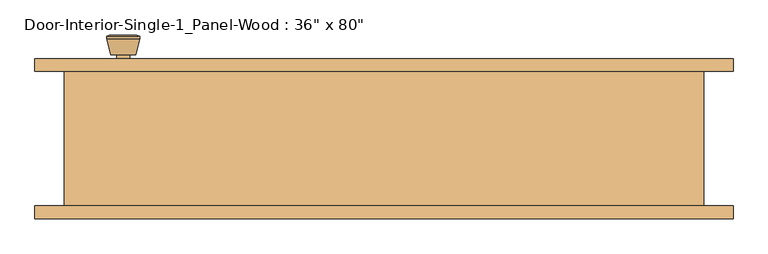
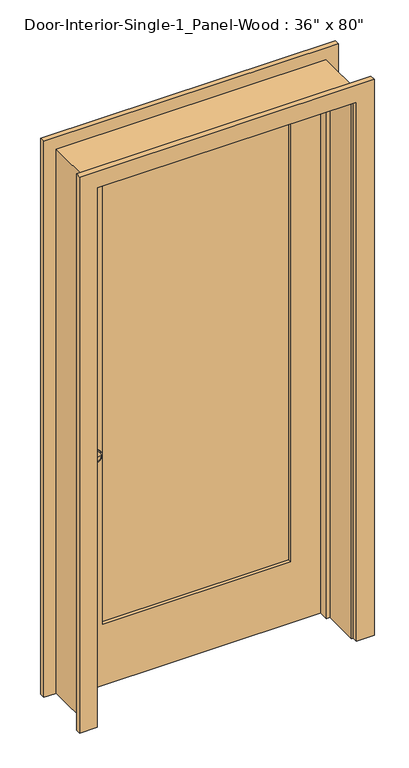
"""IFC4 building model written with IfcOpenShell, lengths in millimetres: door geometry."""

from ifc_helpers import new_model, si_unit, point, frame, frame_2d, origin, place, context, project, spatial, polyline, circle_curve, trimmed, segment, composite_curve, outline, extrude, faceted_brep, source, transform, mapped, element, save
from ifc_brep_helpers import plane_surface, cylinder_surface, revolved_surface, advanced_brep


def door_82825f5f(model_context):
    return source(origin(), model_context, "Body", "SolidModel", [
        advanced_brep(
        [(-393.7, 57.5, 914.4), (-383.7, 57.5, 914.4), (-403.7, 57.5, 914.4), (-373.2241324, 8.5, 914.4), (-393.7, 8.5, 914.4), (-414.1758676, 8.5, 914.4), (-368.7, 10.3278681, 914.4), (-418.7, 10.3278681, 914.4), (-368.7, 13.7915463, 914.4), (-418.7, 13.7915463, 914.4), (-375.063764, 38.5, 914.4), (-412.336236, 38.5, 914.4), (-383.7, 38.5, 914.4), (-403.7, 38.5, 914.4)],
        [
            (0, 1),
            (1, 2, circle_curve(frame((-393.7, 57.5, 914.4), z_axis=(0.0, 1.0, 0.0), x_axis=(-1.0, 0.0, 0.0)), 10.0)),
            (2, 0),
            (2, 1, circle_curve(frame((-393.7, 57.5, 914.4), z_axis=(0.0, 1.0, 0.0), x_axis=(-1.0, 0.0, 0.0)), 10.0)),
            (3, 4),
            (4, 5),
            (5, 3, circle_curve(frame((-393.7, 8.5, 914.4), z_axis=(0.0, -1.0, 0.0), x_axis=(-1.0, 0.0, 0.0)), 20.4758676)),
            (3, 5, circle_curve(frame((-393.7, 8.5, 914.4), z_axis=(0.0, -1.0, 0.0), x_axis=(-1.0, 0.0, 0.0)), 20.4758676)),
            (6, 3),
            (5, 7),
            (7, 6, circle_curve(frame((-393.7, 10.3278681, 914.4), z_axis=(0.0, -1.0, 0.0), x_axis=(-1.0, 0.0, 0.0)), 25.0)),
            (6, 7, circle_curve(frame((-393.7, 10.3278681, 914.4), z_axis=(0.0, -1.0, 0.0), x_axis=(-1.0, 0.0, 0.0)), 25.0)),
            (8, 6),
            (7, 9),
            (9, 8, circle_curve(frame((-393.7, 13.7915463, 914.4), z_axis=(0.0, -1.0, 0.0), x_axis=(-1.0, 0.0, 0.0)), 25.0)),
            (8, 9, circle_curve(frame((-393.7, 13.7915463, 914.4), z_axis=(0.0, -1.0, 0.0), x_axis=(-1.0, 0.0, 0.0)), 25.0)),
            (10, 8),
            (9, 11),
            (11, 10, circle_curve(frame((-393.7, 38.5, 914.4), z_axis=(0.0, -1.0, 0.0), x_axis=(-1.0, 0.0, 0.0)), 18.636236)),
            (10, 11, circle_curve(frame((-393.7, 38.5, 914.4), z_axis=(0.0, -1.0, 0.0), x_axis=(-1.0, 0.0, 0.0)), 18.636236)),
            (12, 10),
            (11, 13),
            (13, 12, circle_curve(frame((-393.7, 38.5, 914.4), z_axis=(0.0, -1.0, 0.0), x_axis=(-1.0, 0.0, 0.0)), 10.0)),
            (12, 13, circle_curve(frame((-393.7, 38.5, 914.4), z_axis=(0.0, -1.0, 0.0), x_axis=(-1.0, 0.0, 0.0)), 10.0)),
            (1, 12),
            (13, 2),
        ],
        [
            plane_surface(frame((-393.7, 57.5, 914.4), z_axis=(0.0, 1.0, 0.0), x_axis=(-1.0, 0.0, 0.0))),
            plane_surface(frame((-393.7, 8.5, 914.4), z_axis=(0.0, -1.0, 0.0), x_axis=(-1.0, 0.0, 0.0))),
            revolved_surface(polyline([(-414.1758676, 8.5, 914.4), (-418.7, 10.3278681, 914.4)]), (-393.7, 57.5, 914.4), (0.0, 1.0, 0.0)),
            cylinder_surface(frame((-393.7, 57.5, 914.4), z_axis=(0.0, 1.0, 0.0), x_axis=(-1.0, 0.0, 0.0)), 25.0),
            revolved_surface(polyline([(-418.7, 13.7915463, 914.4), (-412.336236, 38.5, 914.4)]), (-393.7, 57.5, 914.4), (0.0, 1.0, 0.0)),
            plane_surface(frame((-393.7, 38.5, 914.4), z_axis=(0.0, 1.0, 0.0), x_axis=(-1.0, 0.0, 0.0))),
            cylinder_surface(frame((-393.7, 57.5, 914.4), z_axis=(0.0, 1.0, 0.0), x_axis=(-1.0, 0.0, 0.0)), 10.0),
        ],
        [
            (0, [[1, 2, 3]]),
            (0, [[-3, 4, -1]]),
            (1, [[5, 6, 7]]),
            (1, [[-6, -5, 8]]),
            (2, [[9, -7, 10, 11]]),
            (2, [[-10, -8, -9, 12]]),
            (3, [[13, -11, 14, 15]]),
            (3, [[-14, -12, -13, 16]]),
            (4, [[17, -15, 18, 19]]),
            (4, [[-18, -16, -17, 20]]),
            (5, [[21, -19, 22, 23]]),
            (5, [[-22, -20, -21, 24]]),
            (6, [[25, -23, 26, -2]]),
            (6, [[-26, -24, -25, -4]]),
        ],
    ),
        extrude(outline(composite_curve([segment(trimmed(circle_curve(frame_2d((914.4, -393.7)), 30.0), [point((914.4, -423.7))], [point((914.4, -363.7))], False, "CARTESIAN"), True, "CONTINUOUS"), segment(trimmed(circle_curve(frame_2d((914.4, -393.7)), 30.0), [point((914.4, -363.7))], [point((914.4, -423.7))], False, "CARTESIAN"), True, "CONTINUOUS")], self_intersect=False)), frame((0.0, 57.5, 0.0), z_axis=(0.0, 1.0, 0.0), x_axis=(0.0, 0.0, 1.0)), (0.0, 0.0, 1.0), 6.0),
        advanced_brep(
        [(-393.7, 104.425, 914.4), (-403.7, 104.425, 914.4), (-383.7, 104.425, 914.4), (-373.2241324, 153.425, 914.4), (-414.1758676, 153.425, 914.4), (-393.7, 153.425, 914.4), (-368.7, 151.5971319, 914.4), (-418.7, 151.5971319, 914.4), (-368.7, 148.1334537, 914.4), (-418.7, 148.1334537, 914.4), (-375.063764, 123.425, 914.4), (-412.336236, 123.425, 914.4), (-383.7, 123.425, 914.4), (-403.7, 123.425, 914.4)],
        [
            (0, 1),
            (1, 2, circle_curve(frame((-393.7, 104.425, 914.4), z_axis=(0.0, -1.0, 0.0), x_axis=(-1.0, 0.0, 0.0)), 10.0)),
            (2, 0),
            (2, 1, circle_curve(frame((-393.7, 104.425, 914.4), z_axis=(0.0, -1.0, 0.0), x_axis=(-1.0, 0.0, 0.0)), 10.0)),
            (3, 4, circle_curve(frame((-393.7, 153.425, 914.4), z_axis=(0.0, 1.0, 0.0), x_axis=(-1.0, 0.0, 0.0)), 20.4758676)),
            (4, 5),
            (5, 3),
            (4, 3, circle_curve(frame((-393.7, 153.425, 914.4), z_axis=(0.0, 1.0, 0.0), x_axis=(-1.0, 0.0, 0.0)), 20.4758676)),
            (6, 7, circle_curve(frame((-393.7, 151.5971319, 914.4), z_axis=(0.0, 1.0, 0.0), x_axis=(-1.0, 0.0, 0.0)), 25.0)),
            (7, 4),
            (3, 6),
            (7, 6, circle_curve(frame((-393.7, 151.5971319, 914.4), z_axis=(0.0, 1.0, 0.0), x_axis=(-1.0, 0.0, 0.0)), 25.0)),
            (8, 9, circle_curve(frame((-393.7, 148.1334537, 914.4), z_axis=(0.0, 1.0, 0.0), x_axis=(-1.0, 0.0, 0.0)), 25.0)),
            (9, 7),
            (6, 8),
            (9, 8, circle_curve(frame((-393.7, 148.1334537, 914.4), z_axis=(0.0, 1.0, 0.0), x_axis=(-1.0, 0.0, 0.0)), 25.0)),
            (10, 11, circle_curve(frame((-393.7, 123.425, 914.4), z_axis=(0.0, 1.0, 0.0), x_axis=(-1.0, 0.0, 0.0)), 18.636236)),
            (11, 9),
            (8, 10),
            (11, 10, circle_curve(frame((-393.7, 123.425, 914.4), z_axis=(0.0, 1.0, 0.0), x_axis=(-1.0, 0.0, 0.0)), 18.636236)),
            (12, 13, circle_curve(frame((-393.7, 123.425, 914.4), z_axis=(0.0, 1.0, 0.0), x_axis=(-1.0, 0.0, 0.0)), 10.0)),
            (13, 11),
            (10, 12),
            (13, 12, circle_curve(frame((-393.7, 123.425, 914.4), z_axis=(0.0, 1.0, 0.0), x_axis=(-1.0, 0.0, 0.0)), 10.0)),
            (1, 13),
            (12, 2),
        ],
        [
            plane_surface(frame((-393.7, 104.425, 914.4), z_axis=(0.0, -1.0, 0.0), x_axis=(-1.0, 0.0, 0.0))),
            plane_surface(frame((-393.7, 153.425, 914.4), z_axis=(0.0, 1.0, 0.0), x_axis=(-1.0, 0.0, 0.0))),
            revolved_surface(polyline([(-414.1758676, 153.425, 914.4), (-418.7, 151.5971319, 914.4)]), (-393.7, 104.425, 914.4), (0.0, -1.0, 0.0)),
            cylinder_surface(frame((-393.7, 104.425, 914.4), z_axis=(0.0, -1.0, 0.0), x_axis=(-1.0, 0.0, 0.0)), 25.0),
            revolved_surface(polyline([(-418.7, 148.1334537, 914.4), (-412.336236, 123.425, 914.4)]), (-393.7, 104.425, 914.4), (0.0, -1.0, 0.0)),
            plane_surface(frame((-393.7, 123.425, 914.4), z_axis=(0.0, -1.0, 0.0), x_axis=(-1.0, 0.0, 0.0))),
            cylinder_surface(frame((-393.7, 104.425, 914.4), z_axis=(0.0, -1.0, 0.0), x_axis=(-1.0, 0.0, 0.0)), 10.0),
        ],
        [
            (0, [[1, 2, 3]]),
            (0, [[-3, 4, -1]]),
            (1, [[5, 6, 7]]),
            (1, [[8, -7, -6]]),
            (2, [[9, 10, -5, 11]]),
            (2, [[12, -11, -8, -10]]),
            (3, [[13, 14, -9, 15]]),
            (3, [[16, -15, -12, -14]]),
            (4, [[17, 18, -13, 19]]),
            (4, [[20, -19, -16, -18]]),
            (5, [[21, 22, -17, 23]]),
            (5, [[24, -23, -20, -22]]),
            (6, [[-2, 25, -21, 26]]),
            (6, [[-4, -26, -24, -25]]),
        ],
    ),
        extrude(outline(composite_curve([segment(trimmed(circle_curve(frame_2d((914.4, -393.7)), 30.0), [point((914.4, -423.7))], [point((914.4, -363.7))], False, "CARTESIAN"), True, "CONTINUOUS"), segment(trimmed(circle_curve(frame_2d((914.4, -393.7)), 30.0), [point((914.4, -363.7))], [point((914.4, -423.7))], False, "CARTESIAN"), True, "CONTINUOUS")], self_intersect=False)), frame((0.0, 98.425, 0.0), z_axis=(0.0, 1.0, 0.0), x_axis=(0.0, 0.0, 1.0)), (0.0, 0.0, 1.0), 6.0),
        faceted_brep([(482.6, 98.425, 0.0), (482.6, -104.775, 0.0), (457.2, -104.775, 0.0), (457.2, 28.575, 0.0), (444.5, 28.575, 0.0), (444.5, 63.5, 0.0), (457.2, 63.5, 0.0), (457.2, 98.425, 0.0), (482.6, 98.425, 2057.4), (482.6, -104.775, 2057.4), (-482.6, -104.775, 2057.4), (-482.6, -104.775, 0.0), (-457.2, -104.775, 0.0), (-457.2, -104.775, 2032.0), (457.2, -104.775, 2032.0), (457.2, 28.575, 2032.0), (-457.2, 28.575, 2032.0), (-457.2, 28.575, 0.0), (-444.5, 28.575, 0.0), (-444.5, 28.575, 2019.3), (444.5, 28.575, 2019.3), (444.5, 63.5, 2019.3), (-444.5, 63.5, 2019.3), (-444.5, 63.5, 0.0), (-457.2, 63.5, 0.0), (-457.2, 63.5, 2032.0), (457.2, 63.5, 2032.0), (457.2, 98.425, 2032.0), (-457.2, 98.425, 2032.0), (-457.2, 98.425, 0.0), (-482.6, 98.425, 0.0), (-482.6, 98.425, 2057.4)], [[[0, 1, 2, 3, 4, 5, 6, 7]], [[1, 0, 8, 9]], [[2, 1, 9, 10, 11, 12, 13, 14]], [[3, 2, 14, 15]], [[4, 3, 15, 16, 17, 18, 19, 20]], [[5, 4, 20, 21]], [[6, 5, 21, 22, 23, 24, 25, 26]], [[7, 6, 26, 27]], [[0, 7, 27, 28, 29, 30, 31, 8]], [[9, 8, 31, 10]], [[15, 14, 13, 16]], [[21, 20, 19, 22]], [[27, 26, 25, 28]], [[30, 29, 24, 23, 18, 17, 12, 11]], [[10, 31, 30, 11]], [[16, 13, 12, 17]], [[22, 19, 18, 23]], [[28, 25, 24, 29]]]),
        extrude(outline(polyline([(2032.0, -457.2), (0.0, -457.2), (0.0, 457.2), (2032.0, 457.2), (2032.0, -457.2)]), holes=[polyline([(1912.9375, -336.55), (1912.9375, 336.55), (231.775, 336.55), (231.775, -336.55), (1912.9375, -336.55)])]), frame((0.0, 63.5, 0.0), z_axis=(0.0, 1.0, 0.0), x_axis=(0.0, 0.0, 1.0)), (0.0, 0.0, 1.0), 34.925),
        extrude(outline(polyline([(336.55, 75.1416667), (-336.55, 75.1416667), (-336.55, 86.7833333), (336.55, 86.7833333), (336.55, 75.1416667)])), frame((0.0, 0.0, 231.775), z_axis=(0.0, 0.0, 1.0), x_axis=(1.0, 0.0, 0.0)), (0.0, 0.0, 1.0), 1681.1625),
        extrude(outline(polyline([(0.0, 463.55), (0.0, 527.05), (2101.85, 527.05), (2101.85, -527.05), (0.0, -527.05), (0.0, -463.55), (2038.35, -463.55), (2038.35, 463.55), (0.0, 463.55)])), frame((0.0, 98.425, 0.0), z_axis=(0.0, 1.0, 0.0), x_axis=(0.0, 0.0, 1.0)), (0.0, 0.0, 1.0), 19.05),
        extrude(outline(polyline([(0.0, 463.55), (0.0, 527.05), (2101.85, 527.05), (2101.85, -527.05), (0.0, -527.05), (0.0, -463.55), (2038.35, -463.55), (2038.35, 463.55), (0.0, 463.55)])), frame((0.0, -123.825, 0.0), z_axis=(0.0, 1.0, 0.0), x_axis=(0.0, 0.0, 1.0)), (0.0, 0.0, 1.0), 19.05),
    ])


if __name__ == "__main__":
    model = new_model("IFC4")
    model_context = context("Model", 3, world=origin())
    ifc_project = project(units=[si_unit("LENGTHUNIT", "METRE", prefix="MILLI")], contexts=[model_context])
    site = spatial("IfcSite", under=ifc_project)
    building = spatial("IfcBuilding", under=site)
    placement = place(None, origin())
    door_shape = door_82825f5f(model_context)
    element("IfcDoor", 1, ObjectType="Door-Interior-Single-1_Panel-Wood : 36\" x 80\"", at=placement, inside=building, context=model_context, shape_type="MappedRepresentation", body=[
        mapped(door_shape, transform((0.0, 0.0, 0.0), x_axis=(1.0, 0.0, 0.0), y_axis=(0.0, 1.0, 0.0), z_axis=(0.0, 0.0, 1.0))),
    ])
    save(model, "model.ifc")

# Revit data of these elements
# Type "Door-Interior-Single-1_Panel-Wood : 36\" x 80\""
#   Type Mark = "10"
#   Assembly Code = "C1020300"
#   Analytic Construction = "Wooden"
#   Top Rail = 0' - 4 11/16"
#   Thickness = 0' - 1 3/8"
#   Thermal Resistance (R) = 2.5876 (h·ft²·°F)/BTU
#   Swing Angle [instance default] = 90.00°
#   Stiles = 0' - 4 3/4"
#   Rough Width = 3' - 2"
#   Rough Height = 6' - 9"
#   Height = 6' - 8"
#   Width = 3' - 0"
#   Heat Transfer Coefficient (U) = 0.3865 BTU/(h·ft²·°F)
#   Bottom Rail = 0' - 9 1/8"
#   Trim Material = Cherry
#   Panel Material = Cherry
#   Frame Material = Cherry
#   Door Handle Material = Aluminum
#   Visual Light Transmittance = 0
#   Solar Heat Gain Coefficient = 0
#   Wall Closure = (empty or 0)
#   Function = (empty or 0)
# Element 1 (IfcDoor, "Door-Interior-Single-1_Panel-Wood : 36\" x 80\"")
#   Materials on its faces: "Cherry", "Aluminum"
# Materials
#   "Cherry": class "Wood", colour RGB 226 177 128, transparency 0, Description = "Prunus Serotina", Cost = 0
#   "Aluminum": class "Metal", colour RGB 247 247 247, transparency 0, Description = "Aluminum 6061", Cost = 0
